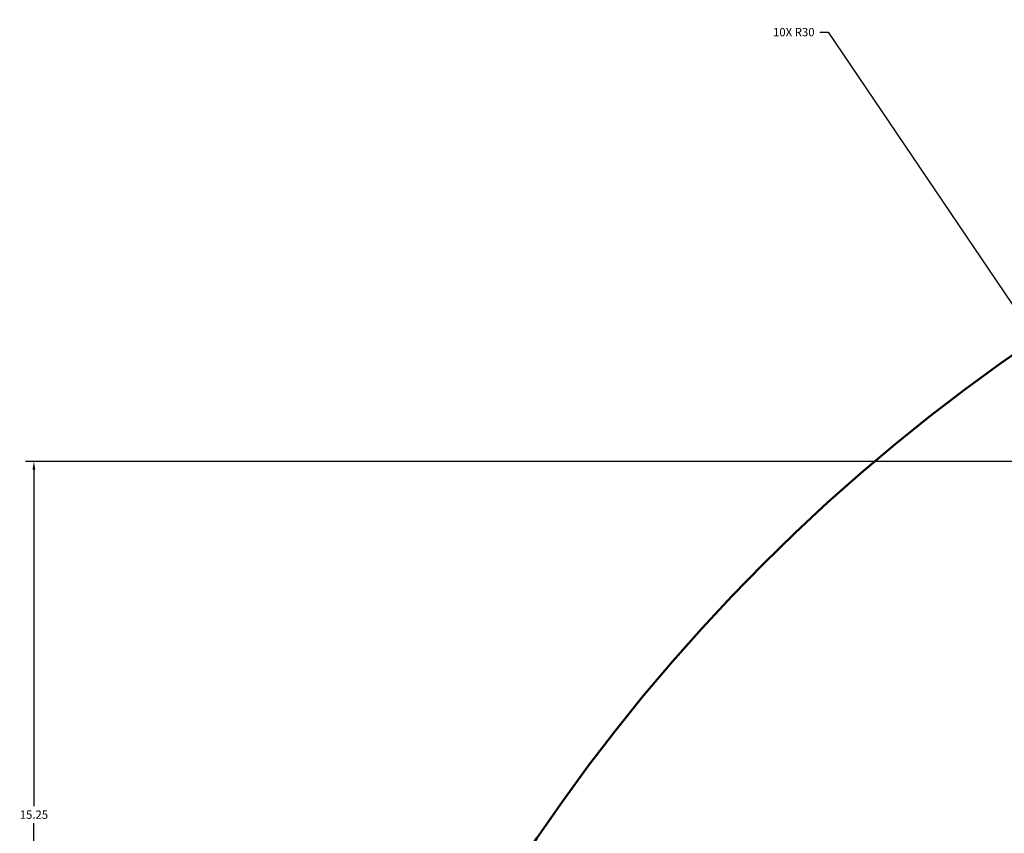
# Model space of a CAD drawing. Units: inches. Extents: x -19.9 to 72.3, y -39.8 to 57.5.
# Tile 6 of 8: x -16.3 to 5, y 35.8 to 53.4. Entities that reach past the tile are written whole.
import ezdxf

# ---------------------------------------------------------------- set-up
doc = ezdxf.new("R2010")
doc.units = ezdxf.units.IN
doc.header["$MEASUREMENT"] = 0
doc.layers.add('M-DIMS', color=2, linetype='Continuous', lineweight=18)
doc.layers.add('M-OUTL', color=7, linetype='Continuous', lineweight=50)
doc.styles.get("Standard").update_dxf_attribs({"font": 'arial.ttf'})
doc.dimstyles.get("Standard").update_dxf_attribs({"dimtxt": 0.18, "dimasz": 0.18, "dimexe": 0.18, "dimexo": 0.0625, "dimgap": 0.09, "dimtad": 0, "dimtih": 1, "dimtoh": 1, "dimdec": 4, "dimzin": 0, "dimdsep": 46, "dimtxsty": 'Standard', "dimcen": 0.09, "dimadec": 0, "dimazin": 0, "dimtfac": 1, "dimtdec": 4, "dimtofl": 0, "dimtmove": 0, "dimatfit": 3, "dimfxl": 1, "dimtolj": 1, "dimtzin": 0, "dimarcsym": 0})

# ---------------------------------------------------------------- blocks, each defined once
blk = doc.blocks.new('*D10')
at = {"layer": 'Defpoints', "color": 0, "transparency": 16777216}
for p in [(28.06, 43.841), (-15.966, 28.591), (1.646, 28.591)]:
    blk.add_point(p, dxfattribs=at)
at = {"layer": 'M-DIMS', "color": 0, "lineweight": -2, "transparency": 16777216}
for p, q in [((27.997, 43.841), (-16.146, 43.841)), ((-15.966, 43.661), (-15.966, 36.398)), ((-15.966, 28.771), (-15.966, 36.034)), ((1.584, 28.591), (-16.146, 28.591))]:
    blk.add_line(p, q, dxfattribs=at)
at = {"layer": 'M-DIMS', "color": 0, "transparency": 16777216}
for points in [[(-15.996, 43.661), (-15.936, 43.661), (-15.966, 43.841)], [(-15.996, 28.771), (-15.936, 28.771), (-15.966, 28.591)]]:
    blk.add_solid(points, dxfattribs=at)
at = {"layer": 'M-DIMS', "color": 0, "transparency": 16777216, "insert": (-15.966, 36.216), "char_height": 0.18, "attachment_point": 5}
blk.add_mtext('\\A1;15.25', dxfattribs=at)
blk = doc.blocks.new('*D13')
at = {"layer": 'Defpoints', "color": 0, "transparency": 16777216}
for p in [(11.256, 38.194), (28.06, 13.341)]:
    blk.add_point(p, dxfattribs=at)
at = {"layer": 'M-DIMS', "color": 0, "lineweight": -2, "transparency": 16777216}
for p, q in [((0.994, 53.105), (1.174, 53.105)), ((1.174, 53.105), (11.155, 38.343)), ((28.06, 13.251), (28.06, 13.431)), ((27.97, 13.341), (28.15, 13.341))]:
    blk.add_line(p, q, dxfattribs=at)
at = {"layer": 'M-DIMS', "color": 0, "transparency": 16777216}
blk.add_solid([(11.18, 38.36), (11.131, 38.326), (11.256, 38.194)], dxfattribs=at)
at = {"layer": 'M-DIMS', "color": 0, "transparency": 16777216, "insert": (0.434, 53.105), "char_height": 0.18, "attachment_point": 5}
blk.add_mtext('\\A1;10X R30', dxfattribs=at)

msp = doc.modelspace()

# ---------------------------------------------------------------- linework, layer by layer
at = {"layer": 'M-OUTL'}
msp.add_circle((28.06, 13.341), 40, dxfattribs=at)

# ---------------------------------------------------------------- dimensions: what is measured, and where the dimension line sits
at = {"layer": 'M-DIMS'}
dim = msp.add_radius_dim(center=(28.06, 13.341), mpoint=(11.256, 38.194), text='10X <>', dimstyle='Standard', override={"dimdec": 0, "dimlfac": 1, "dimrnd": 0, "dimzin": 0, "dimdsep": 46, "dimlunit": 2}, dxfattribs=at)
dim.commit()
dim.dimension.update_dxf_attribs({"geometry": '*D13', "text_midpoint": (0.434, 53.105), "dimtype": 164})
dim = msp.add_linear_dim(base=(-15.966, 28.591), p1=(28.06, 43.841), p2=(1.646, 28.591), angle=90, dimstyle='Standard', override={"dimdec": 2, "dimlfac": 1, "dimrnd": 0, "dimzin": 0, "dimdsep": 46, "dimlunit": 2}, dxfattribs=at)
dim.commit()
dim.dimension.update_dxf_attribs({"geometry": '*D10', "text_midpoint": (-15.966, 36.216)})

doc.saveas('drawing.dxf')
